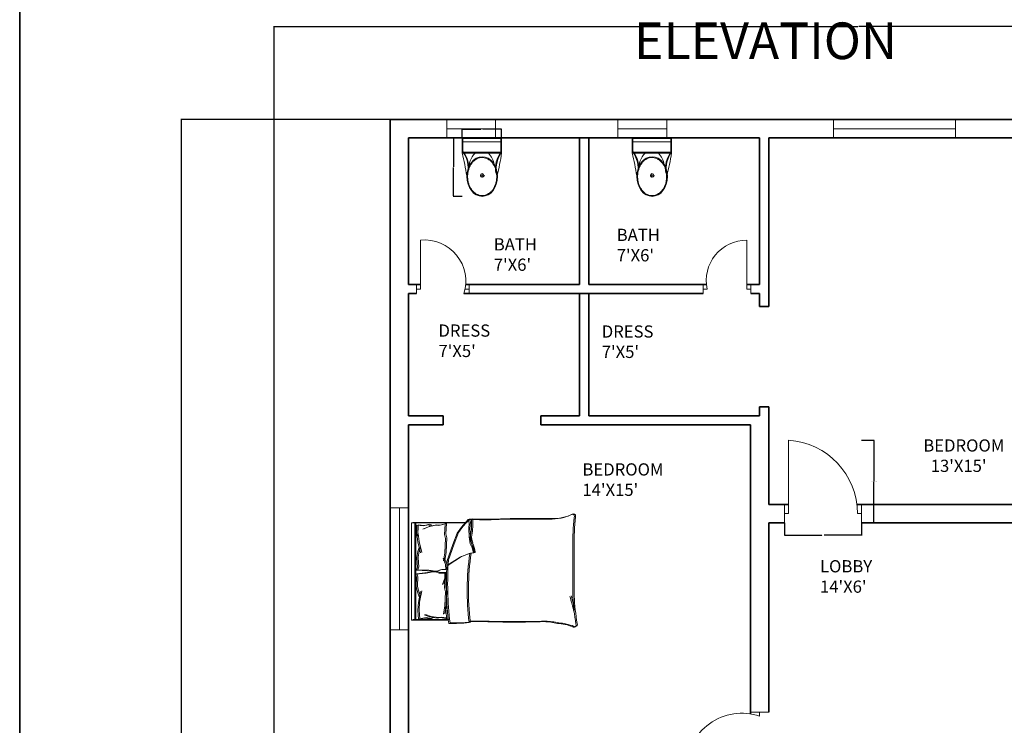
# Model space of a CAD drawing. Units: inches. Extents: x 1824 to 3509, y 619 to 2294.
# Tile 6 of 12: x 1824 to 2308, y 1325 to 1671. Entities that reach past the tile are written whole.
import ezdxf

# ---------------------------------------------------------------- set-up
doc = ezdxf.new("R2010")
doc.units = ezdxf.units.IN
for name, color, linetype, lineweight in [('A-ANNO-DIMS', 2, 'Continuous', 18), ('A-ANNO-TEXT', 7, 'Continuous', 25), ('A-ANNO-TTLB', 7, 'Continuous', 35), ('A-AREA-IDEN', 7, 'Continuous', 18), ('A-DOOR', 3, 'Continuous', 18), ('A-FLOR-FIXT', 9, 'Continuous', 18), ('A-FURN', 8, 'Continuous', 13), ('A-GLAZ', 4, 'Continuous', 18), ('A-WALL', 7, 'Continuous', 35)]:
    doc.layers.add(name, color=color, linetype=linetype, lineweight=lineweight)
doc.styles.get("Standard").update_dxf_attribs({"font": 'arial.ttf'})
doc.dimstyles.get("Standard").update_dxf_attribs({"dimtxt": 0.18, "dimasz": 0.18, "dimexe": 0.18, "dimexo": 0.0625, "dimgap": 0.09, "dimtad": 0, "dimtih": 1, "dimtoh": 1, "dimdec": 4, "dimzin": 0, "dimdsep": 46, "dimtxsty": 'Standard', "dimcen": 0.09, "dimadec": 0, "dimazin": 0, "dimtfac": 1, "dimtdec": 4, "dimtofl": 0, "dimtmove": 0, "dimatfit": 3, "dimfxl": 1, "dimtolj": 1, "dimtzin": 0, "dimarcsym": 0})

# ---------------------------------------------------------------- blocks, each defined once
blk = doc.blocks.new('A$C31115884')
for p, q in [((258, 466), (258, 523)), ((283, 498), (223, 498)), ((0, 200), (0, 0)), ((520, 200), (0, 200)), ((10, 190), (10, 10)), ((510, 190), (10, 190)), ((510, 10), (510, 190)), ((520, 0), (520, 200)), ((510, 54), (0, 54)), ((10, 10), (510, 10)), ((0, 0), (520, 0))]:
    blk.add_line(p, q)
blk.add_circle((256, 496), 23.6)
for centre, radius, start, end in [((2778, -205), 2807, 165.4549, 171.7133), ((-295, 403), 365, 324.2091, 9.3499), ((-295, 403), 375, 324.2091, 9.3499), ((139, 406), 293, 315.8436, 2.6563), ((806, 403), 375, 179.2036, 215.7909), ((806, 403), 365, 170.6501, 215.7909), ((3237, 905), 2807, 188.2867, 194.5451), ((384, 406), 293, 190.2774, 224.1564)]:
    blk.add_arc(centre, radius, start, end)
blk.add_ellipse((256, 510), major_axis=(0, -261), ratio=0.772727)
blk.add_open_spline([(256, 259), (263, 259), (270, 260), (288, 262), (299, 265), (320, 273), (330, 278), (350, 291), (360, 299), (378, 316), (386, 326), (402, 347), (409, 358), (421, 383), (427, 395), (436, 422), (440, 436), (445, 465), (447, 480), (448, 509), (448, 524), (445, 553), (443, 568), (436, 596), (432, 610), (422, 636), (416, 649), (402, 672), (395, 683), (379, 703), (370, 712), (351, 728), (341, 735), (321, 746), (310, 751), (289, 757), (278, 759), (256, 761), (245, 761), (223, 757), (212, 754), (191, 746), (181, 741), (161, 728), (151, 720), (133, 703), (125, 693), (110, 672), (103, 660), (90, 636), (85, 623), (76, 596), (72, 582), (67, 553), (66, 538), (64, 509), (65, 494), (68, 465), (70, 450), (77, 422), (81, 408), (91, 382), (97, 370), (111, 346), (118, 335), (135, 316), (144, 307), (162, 291), (172, 284), (193, 273), (203, 269), (225, 262), (236, 260), (250, 259), (253, 259), (256, 259)], degree=3, knots=[0, 0, 0, 0, 0.110105, 0.110105, 0.285049, 0.285049, 0.459994, 0.459994, 0.634938, 0.634938, 0.809882, 0.809882, 0.984827, 0.984827, 1.159771, 1.159771, 1.334715, 1.334715, 1.50966, 1.50966, 1.684604, 1.684604, 1.859549, 1.859549, 2.034493, 2.034493, 2.209437, 2.209437, 2.384382, 2.384382, 2.559326, 2.559326, 2.73427, 2.73427, 2.909215, 2.909215, 3.084159, 3.084159, 3.259103, 3.259103, 3.434048, 3.434048, 3.608992, 3.608992, 3.783936, 3.783936, 3.958881, 3.958881, 4.133825, 4.133825, 4.30877, 4.30877, 4.483714, 4.483714, 4.658658, 4.658658, 4.833603, 4.833603, 5.008547, 5.008547, 5.183491, 5.183491, 5.358436, 5.358436, 5.53338, 5.53338, 5.708324, 5.708324, 5.883269, 5.883269, 6.058213, 6.058213, 6.233158, 6.233158, 6.283185, 6.283185, 6.283185, 6.283185])
blk = doc.blocks.new('DOOR-BATH-W-24')
for p, q in [((2, 2.25), (2, 26.25)), ((0, 4.5), (0, 0)), ((0, 0), (0, 2.25)), ((0, 2.25), (2, 2.25)), ((25.84, 2.25), (23.84, 2.25)), ((25.84, 4.5), (25.84, 0)), ((25.84, 0), (25.84, 2.25))]:
    blk.add_line(p, q)
blk.add_arc((4.03, 6.16), 20.2, 342.2542, 95.7568)
blk = doc.blocks.new('DOOR-BATH-C-24')
for p, q in [((21.44, 2.25), (21.44, 26.25)), ((0, 4.5), (0, 0)), ((0, 0), (0, 2.25)), ((0, 2.25), (2, 2.25)), ((23.44, 2.25), (21.44, 2.25)), ((23.44, 4.5), (23.44, 0)), ((23.44, 0), (23.44, 2.25))]:
    blk.add_line(p, q)
blk.add_arc((21.44, 6.38), 19.87, 90, 191.9846)
blk = doc.blocks.new('DOOR-BED-W-36')
for p, q in [((31.5, 29.8), (40.5, 29.8)), ((40.5, 29.8), (36, 29.8)), ((36, 29.8), (36, 27.8)), ((36, 2), (0, 2)), ((31.5, 0), (31.5, 0)), ((31.5, 0), (40.5, 0)), ((36, 0), (36, 2)), ((40.5, 0), (36, 0)), ((36, 0), (36, 0)), ((40.5, 0), (40.5, 0))]:
    blk.add_line(p, q)
blk.add_arc((27.25, 2), 27.25, 71.2585, 180)
blk = doc.blocks.new('DOOR-BED-C-36')
for p, q in [((2, 4.5), (2, 40.5)), ((0, 9), (0, 0)), ((37.83, 9), (37.83, 9)), ((37.83, 9), (37.83, 0)), ((0, 0), (0, 4.5)), ((0, 4.5), (2, 4.5)), ((37.83, 4.5), (35.83, 4.5)), ((37.83, 0), (37.83, 4.5))]:
    blk.add_line(p, q)
blk.add_arc((-0.24, 4.5), 36.07, 0, 86.4439)
blk = doc.blocks.new('BED-DOUBLE-PLAN')
for p, q in [((0, 51.27), (26.61, 51.27)), ((0, 51.27), (26.61, 51.27)), ((0, 3.48), (0, 51.27)), ((0.64, 51.49), (27.25, 51.49)), ((0.64, 51.49), (27.25, 51.49)), ((1.53, 3.48), (1.53, 51.27)), ((1.53, 3.48), (1.53, 51.27)), ((2.17, 3.7), (2.17, 51.49)), ((2.17, 3.7), (2.17, 51.49)), ((2.56, 50.11), (2.46, 44.71)), ((2.56, 50.11), (2.46, 44.71)), ((2.56, 50.11), (5.77, 49.73)), ((2.56, 50.11), (5.77, 49.73)), ((3.2, 50.34), (3.1, 44.94)), ((3.2, 50.34), (3.1, 44.94)), ((3.2, 50.34), (6.41, 49.96)), ((3.2, 50.34), (6.41, 49.96)), ((8.26, 49.31), (5.58, 48.13)), ((8.26, 49.31), (5.58, 48.13)), ((5.77, 49.73), (8.34, 50.33)), ((5.77, 49.73), (8.34, 50.33)), ((8.9, 49.54), (6.22, 48.36)), ((8.9, 49.54), (6.22, 48.36)), ((6.41, 49.96), (8.98, 50.56)), ((6.41, 49.96), (8.98, 50.56)), ((11.83, 50.11), (8.26, 49.31)), ((11.83, 50.11), (8.26, 49.31)), ((8.34, 50.33), (9.38, 49.82)), ((8.34, 50.33), (9.38, 49.81)), ((12.47, 50.34), (8.9, 49.54)), ((12.47, 50.34), (8.9, 49.54)), ((8.98, 50.56), (10.02, 50.04)), ((8.98, 50.56), (10.02, 50.04)), ((13.43, 49.92), (11.83, 50.11)), ((13.43, 49.92), (11.83, 50.11)), ((14.07, 50.15), (12.47, 50.34)), ((14.07, 50.15), (12.47, 50.34)), ((16.57, 50.7), (13.43, 49.92)), ((16.57, 50.7), (13.43, 49.92)), ((17.21, 50.93), (14.07, 50.15)), ((17.21, 50.93), (14.07, 50.15)), ((16.17, 45.57), (16.57, 50.7)), ((16.17, 45.57), (16.57, 50.7)), ((16.81, 45.8), (17.21, 50.93)), ((16.81, 45.8), (17.21, 50.93)), ((24.5, 49.16), (22.33, 46.22)), ((24.5, 49.16), (22.33, 46.22)), ((25.13, 49.39), (22.97, 46.45)), ((25.13, 49.39), (22.97, 46.45)), ((27.75, 52.87), (24.5, 49.16)), ((27.75, 52.87), (24.5, 49.16)), ((28.39, 53.1), (25.13, 49.39)), ((28.39, 53.1), (25.13, 49.39)), ((29.49, 52.95), (27.75, 52.87, 3.87)), ((29.49, 52.95), (27.75, 52.87, 3.87)), ((28.36, 51.33), (27.75, 52.87)), ((28.36, 51.33), (27.75, 52.87)), ((28.06, 48.23), (28.36, 51.33)), ((28.06, 48.23), (28.36, 51.33)), ((30.13, 53.18), (28.39, 53.1, 3.87)), ((30.13, 53.18), (28.39, 53.1, 3.87)), ((29, 51.56), (28.39, 53.1)), ((29, 51.56), (28.39, 53.1)), ((28.69, 48.46), (29, 51.56)), ((28.69, 48.46), (29, 51.56)), ((29, 44.59), (28.69, 48.46)), ((29, 44.59), (28.69, 48.46)), ((2.46, 44.71), (2.54, 45.71)), ((2.46, 44.71), (2.54, 45.71)), ((2.54, 45.71), (3.07, 41.92)), ((2.54, 45.71), (3.07, 41.91)), ((3.1, 44.94), (3.18, 45.94)), ((3.1, 44.94), (3.18, 45.94)), ((3.18, 45.94), (3.71, 42.14)), ((3.18, 45.94), (3.71, 42.14)), ((16.73, 43.61), (16.17, 45.57)), ((16.73, 43.61), (16.17, 45.57)), ((16.3, 36.6), (16.73, 43.61)), ((16.3, 36.6), (16.73, 43.61)), ((17.37, 43.84), (16.81, 45.8)), ((17.37, 43.83), (16.81, 45.8)), ((16.93, 36.83), (17.37, 43.84)), ((16.93, 36.82), (17.37, 43.83)), ((22.33, 46.22), (20.32, 40.64)), ((22.33, 46.22), (20.32, 40.64)), ((22.97, 46.45), (20.96, 40.87)), ((22.97, 46.45), (20.96, 40.87)), ((28.36, 44.36), (28.06, 48.23)), ((28.36, 44.36), (28.06, 48.23)), ((28.83, 40.95), (28.36, 44.36)), ((28.83, 40.95), (28.36, 44.36)), ((29.47, 41.18), (29, 44.59)), ((29.47, 41.18), (29, 44.59)), ((3.07, 41.92), (4.42, 36.5)), ((3.07, 41.91), (4.42, 36.5)), ((3.67, 39.2), (3.08, 37.14)), ((3.67, 39.2), (3.08, 37.14)), ((3.71, 42.14), (5.06, 36.72)), ((3.71, 42.14), (5.06, 36.72)), ((4.31, 39.43), (3.72, 37.36)), ((4.31, 39.43), (3.72, 37.36)), ((20.32, 40.64), (17.38, 32.31)), ((20.32, 40.64), (17.38, 32.31)), ((20.96, 40.87), (18.02, 32.54)), ((20.96, 40.87), (18.02, 32.53)), ((29.76, 38.94), (28.83, 40.95)), ((29.76, 38.94), (28.83, 40.95)), ((30.4, 39.17), (29.47, 41.18)), ((30.4, 39.17), (29.47, 41.18)), ((30.38, 36.46), (29.76, 38.94)), ((30.38, 36.46), (29.76, 38.94)), ((31.02, 36.69), (30.4, 39.17)), ((31.02, 36.69), (30.4, 39.17)), ((79.24, 15.06), (79.24, 39.68)), ((79.24, 15.06), (79.24, 39.68)), ((79.88, 15.29), (79.88, 39.91)), ((79.88, 15.29), (79.88, 39.91)), ((3.08, 37.14), (2.54, 34.21)), ((3.08, 37.14), (2.54, 34.21)), ((2.54, 34.21), (2.56, 33.88)), ((2.54, 34.21), (2.56, 33.88)), ((2.56, 33.88), (2.98, 29.46)), ((2.56, 33.88), (2.98, 29.46)), ((3.72, 37.36), (3.18, 34.43)), ((3.72, 37.36), (3.18, 34.43)), ((3.18, 34.43), (3.2, 34.11)), ((3.18, 34.43), (3.2, 34.11)), ((3.2, 34.11), (3.62, 29.68)), ((3.2, 34.11), (3.62, 29.68)), ((15.63, 32.56), (16.3, 36.6)), ((15.63, 32.56), (16.3, 36.6)), ((17.38, 30.98), (16.09, 34.05)), ((17.38, 30.98), (16.09, 34.05)), ((16.27, 32.79), (16.93, 36.83)), ((16.27, 32.79), (16.93, 36.82)), ((17.38, 30.26), (23.88, 34.45)), ((17.38, 30.26), (23.88, 34.45)), ((18.02, 30.49), (24.52, 34.68)), ((18.02, 30.49), (24.52, 34.68)), ((23.88, 34.45), (28.36, 36.15)), ((23.88, 34.45), (28.36, 36.15)), ((24.52, 34.68), (29, 36.38)), ((24.52, 34.68), (29, 36.38)), ((28.36, 36.15), (30.38, 36.46)), ((28.36, 36.15), (30.38, 36.46)), ((29, 36.38), (31.02, 36.69)), ((29, 36.38), (31.02, 36.69)), ((2.98, 29.46), (2.49, 27.98)), ((2.98, 29.46), (2.49, 27.98)), ((3.62, 29.68), (3.13, 28.21)), ((3.62, 29.68), (3.13, 28.21)), ((16.74, 30.75), (15.45, 33.82)), ((16.74, 30.75), (15.45, 33.82)), ((16.89, 28.3), (16.74, 30.75)), ((16.89, 28.3), (16.74, 30.75)), ((17.53, 28.53), (17.38, 30.98)), ((17.53, 28.53), (17.38, 30.98)), ((1.87, 25.98), (7.22, 26.56)), ((1.87, 25.98), (7.22, 26.56)), ((2.45, 24.54), (1.87, 25.98)), ((2.45, 24.54), (1.87, 25.98)), ((2.3, 20.09), (2.45, 24.54)), ((2.3, 20.09), (2.45, 24.54)), ((2.49, 27.98), (7.87, 27.73)), ((2.49, 27.98), (7.87, 27.73)), ((2.51, 26.21), (7.86, 26.79)), ((2.51, 26.21), (7.86, 26.79)), ((3.09, 24.77), (2.51, 26.21)), ((3.09, 24.77), (2.51, 26.21)), ((2.94, 20.32), (3.09, 24.77)), ((2.94, 20.32), (3.09, 24.77)), ((3.13, 28.21), (8.51, 27.96)), ((3.13, 28.21), (8.51, 27.96)), ((7.22, 26.56), (10.4, 27.14)), ((7.22, 26.56), (10.4, 27.14)), ((7.86, 26.79), (11.04, 27.37)), ((7.86, 26.79), (11.04, 27.37)), ((7.87, 27.73), (11.08, 27.36)), ((7.87, 27.73), (11.08, 27.36)), ((8.51, 27.96), (11.72, 27.58)), ((8.51, 27.96), (11.72, 27.58)), ((10.4, 27.14), (11.7, 27.14)), ((10.4, 27.14), (11.7, 27.14)), ((11.04, 27.37), (12.34, 27.37)), ((11.04, 27.37), (12.34, 27.37)), ((11.08, 27.36), (12.38, 27.44)), ((11.08, 27.36), (12.38, 27.44)), ((11.7, 27.14), (13.58, 26.56)), ((11.7, 27.14), (13.58, 26.56)), ((11.72, 27.58), (13.02, 27.67)), ((11.72, 27.58), (13.02, 27.66)), ((12.34, 27.37), (14.22, 26.79)), ((12.34, 27.37), (14.22, 26.79)), ((12.38, 27.44), (14.22, 28.13)), ((12.38, 27.44), (14.22, 28.13)), ((13.02, 27.67), (14.86, 28.36)), ((13.02, 27.66), (14.86, 28.36)), ((13.58, 26.56), (16.26, 26.56)), ((13.58, 26.56), (16.26, 26.56)), ((14.22, 28.13), (16.89, 28.3)), ((14.22, 28.13), (16.89, 28.3)), ((14.22, 26.79), (16.9, 26.79)), ((14.22, 26.79), (16.9, 26.79)), ((14.86, 28.36), (17.53, 28.53)), ((14.86, 28.36), (17.53, 28.53)), ((16.9, 24.33), (15.81, 21.19)), ((16.9, 24.33), (15.81, 21.19)), ((16.17, 19.38), (16.57, 24.52)), ((16.17, 19.38), (16.57, 24.52)), ((16.26, 26.56), (16.26, 24.1)), ((16.26, 26.56), (16.26, 24.1)), ((16.81, 19.61), (17.21, 24.74)), ((16.81, 19.61), (17.21, 24.74)), ((16.9, 26.79), (16.9, 24.33)), ((16.9, 26.79), (16.9, 24.33)), ((2.3, 19.77), (2.3, 20.09)), ((2.3, 19.77), (2.3, 20.09)), ((3.03, 16.88), (2.3, 19.77)), ((3.03, 16.88), (2.3, 19.77)), ((2.94, 20), (2.94, 20.32)), ((2.94, 20), (2.94, 20.32)), ((3.67, 17.11), (2.94, 20)), ((3.67, 17.11), (2.94, 20)), ((16.26, 24.1), (15.17, 20.96)), ((16.26, 24.1), (15.17, 20.96)), ((16.73, 17.42), (16.17, 19.38)), ((16.73, 17.42), (16.17, 19.38)), ((17.37, 17.65), (16.81, 19.61)), ((17.37, 17.65), (16.81, 19.61)), ((3.75, 14.86), (3.03, 16.88)), ((3.75, 14.86), (3.03, 16.88)), ((3.32, 12.11), (4.33, 17.6)), ((3.32, 12.11), (4.33, 17.6)), ((4.39, 15.08), (3.67, 17.11)), ((4.39, 15.08), (3.67, 17.11)), ((3.96, 12.34), (4.97, 17.83)), ((3.96, 12.34), (4.97, 17.83)), ((16.3, 10.41), (16.73, 17.42)), ((16.3, 10.41), (16.73, 17.42)), ((16.93, 10.64), (17.37, 17.65)), ((16.93, 10.64), (17.37, 17.65)), ((3.03, 8.29), (3.32, 12.11)), ((3.03, 8.29), (3.32, 12.11)), ((3.67, 8.51), (3.96, 12.34)), ((3.67, 8.51), (3.96, 12.34)), ((15.63, 6.38), (16.3, 10.41)), ((15.63, 6.38), (16.3, 10.41)), ((16.27, 6.61), (16.93, 10.64)), ((16.27, 6.61), (16.93, 10.64)), ((16.3, 10.41), (16.62, 9.28)), ((16.3, 10.41), (16.62, 9.28)), ((16.93, 10.64), (17.26, 9.51)), ((16.93, 10.64), (17.26, 9.51)), ((3.01, 8.18), (3.03, 8.29)), ((3.01, 8.18), (3.03, 8.29)), ((3.34, 3.9), (3.01, 8.18)), ((3.34, 3.9), (3.01, 8.18)), ((3.65, 8.41), (3.67, 8.51)), ((3.65, 8.41), (3.67, 8.51)), ((3.98, 4.13), (3.65, 8.41)), ((3.98, 4.13), (3.65, 8.41)), ((8.95, 5.05), (6.21, 6.06)), ((8.95, 5.05), (6.21, 6.06)), ((9.59, 5.28), (6.85, 6.29)), ((9.59, 5.28), (6.85, 6.29)), ((12.57, 4.47), (8.95, 5.05)), ((12.57, 4.47), (8.95, 5.05)), ((13.21, 4.7), (9.59, 5.28)), ((13.21, 4.7), (9.59, 5.28)), ((9.74, 4.27), (10.75, 4.85)), ((9.74, 4.27), (10.75, 4.85)), ((14.8, 4.99), (13.21, 4.7)), ((14.8, 4.99), (13.21, 4.7)), ((17.98, 4.41), (14.8, 4.99)), ((17.98, 4.41), (14.8, 4.99)), ((16.62, 9.28), (17.34, 4.18)), ((16.62, 9.28), (17.34, 4.18)), ((17.26, 9.51), (17.98, 4.41)), ((17.26, 9.51), (17.98, 4.41)), ((18.11, 3.48), (0, 3.48)), ((18.11, 3.48), (0, 3.48)), ((18.75, 3.7), (0.64, 3.7)), ((18.75, 3.7), (0.64, 3.7)), ((3.32, 3.9), (6.5, 4.47)), ((3.32, 3.9), (6.5, 4.47)), ((3.96, 4.12), (7.14, 4.7)), ((3.96, 4.12), (7.14, 4.7)), ((6.5, 4.47), (9.1, 4.04)), ((6.5, 4.47), (9.1, 4.04)), ((7.14, 4.7), (9.74, 4.27)), ((7.14, 4.7), (9.74, 4.27)), ((9.1, 4.04), (10.11, 4.62)), ((9.1, 4.04), (10.11, 4.62)), ((14.16, 4.76), (12.57, 4.47)), ((14.16, 4.76), (12.57, 4.47)), ((17.34, 4.18), (14.16, 4.76)), ((17.34, 4.18), (14.16, 4.76))]:
    blk.add_line(p, q)
for centre, radius, start, end in [((36.95, 182.49), 129.5, 266.9791, 273.8365), ((36.95, 182.49), 129.5, 266.9791, 273.8365), ((68.46, -4508.51), 4561.86, 90.00217, 90.28689), ((68.46, -4508.51), 4561.86, 90.00217, 90.28689), ((68.67, 76.16), 23.07, 267.4714, 296.4681), ((68.67, 76.16), 23.07, 267.4714, 296.4681), ((69.31, 76.39), 23.07, 267.4714, 296.4681), ((69.31, 76.39), 23.07, 267.4714, 296.4681), ((78.87, 54.41), 1.1, 332.6588, 86.02), ((78.87, 54.41), 1.1, 332.6588, 86.02), ((212.28, 41.15), 133.04, 174.4998, 180.6351), ((212.28, 41.15), 133.04, 174.4998, 180.6351), ((79.51, 54.64), 1.1, 332.6588, 86.02), ((79.51, 54.64), 1.1, 332.6588, 86.02), ((212.92, 41.38), 133.04, 174.4998, 180.6351), ((212.92, 41.38), 133.04, 174.4998, 180.6351), ((-6.66, 51.33), 36.18, 349.8763, 2.5657), ((-6.66, 51.33), 36.18, 349.8763, 2.5657), ((36.32, 182.27), 129.5, 266.9791, 273.8365), ((36.32, 182.27), 129.5, 266.9791, 273.8365), ((-6.02, 51.56), 36.18, 349.8763, 2.5657), ((-6.02, 51.56), 36.18, 349.8763, 2.5657), ((67.82, -4508.74), 4561.86, 90.00217, 90.28689), ((67.82, -4508.74), 4561.86, 90.00217, 90.28689), ((35.07, 43.74), 6.22, 168.6608, 203.7384), ((35.07, 43.74), 6.22, 168.6608, 203.7384), ((35.71, 43.97), 6.22, 168.6608, 203.7384), ((35.71, 43.97), 6.22, 168.6608, 203.7384), ((1.48, 31.15), 29.65, 10.6617, 19.8806), ((1.48, 31.15), 29.65, 10.6617, 19.8806), ((2.12, 31.38), 29.65, 10.6617, 19.8806), ((2.12, 31.38), 29.65, 10.6617, 19.8806), ((156.32, 17.76), 129.02, 171.7845, 186.9006), ((156.32, 17.76), 129.02, 171.7845, 186.9006), ((156.96, 17.98), 129.02, 171.7845, 186.9006), ((156.96, 17.98), 129.02, 171.7845, 186.9006), ((30.44, 36.64), 0.185, 250.2464, 1.1377), ((30.44, 36.64), 0.185, 250.2464, 1.1377), ((31.08, 36.87), 0.185, 250.2464, 1.1377), ((31.08, 36.87), 0.185, 250.2464, 1.1377), ((182.05, 21.36), 164.97, 176.0865, 186.7821), ((182.05, 21.36), 164.97, 176.0865, 186.7821), ((182.69, 21.59), 164.97, 176.0865, 186.7821), ((182.69, 21.59), 164.97, 176.0865, 186.7821), ((-23.71, -17.22), 106.46, 13.3832, 17.7053), ((-23.71, -17.22), 106.46, 13.3832, 17.7053), ((-23.07, -16.99), 106.46, 13.3832, 17.7053), ((-23.07, -16.99), 106.46, 13.3832, 17.7053), ((200.84, 21.43), 121.76, 182.9958, 189.4091), ((200.84, 21.43), 121.76, 182.9958, 189.4091), ((201.48, 21.66), 121.76, 182.9958, 189.4091), ((201.48, 21.66), 121.76, 182.9958, 189.4091), ((20.1, 85.16), 83.31, 268.7218, 275.604), ((20.1, 85.16), 83.31, 268.7218, 275.604), ((20.74, 85.39), 83.31, 268.7218, 275.604), ((20.74, 85.39), 83.31, 268.7218, 275.604), ((31.17, -167.31), 170.11, 88.4762, 91.0082), ((31.17, -167.31), 170.11, 88.4762, 91.0082), ((31.81, -167.08), 170.11, 88.4762, 91.0082), ((31.81, -167.08), 170.11, 88.4762, 91.0082), ((50.61, 484.82), 482.31, 268.2277, 271.7185), ((50.61, 484.82), 482.31, 268.2277, 271.7185), ((51.25, 485.05), 482.31, 268.2277, 271.7185), ((51.25, 485.05), 482.31, 268.2277, 271.7185), ((64.52, -26.9), 29.63, 76.0648, 88.9113), ((64.52, -26.9), 29.63, 76.0648, 88.9113), ((65.15, -26.67), 29.63, 76.0648, 88.9113), ((65.15, -26.67), 29.63, 76.0648, 88.9113), ((70.28, -21.66), 23.56, 67.9751, 86.652), ((70.28, -21.66), 23.56, 67.9751, 86.652), ((70.91, -21.43), 23.56, 67.9751, 86.652), ((70.91, -21.43), 23.56, 67.9751, 86.652), ((79.72, 1.09), 1.09, 236.1736, 23.4781), ((79.72, 1.09), 1.09, 236.1736, 23.4781), ((80.36, 1.32), 1.09, 236.1736, 23.4781), ((80.36, 1.32), 1.09, 236.1736, 23.4781)]:
    blk.add_arc(centre, radius, start, end)
blk = doc.blocks.new('WIN-24')
for p, q in [((0, 0), (0, 9)), ((0, 9), (0, 4.5)), ((24, 0), (24, 9)), ((0, 4.5), (24, 4.5)), ((24, 4.5), (24, 0))]:
    blk.add_line(p, q)
blk = doc.blocks.new('WIN-60')
for p, q in [((0, 9), (0, 0)), ((60, 4.5), (60, 9)), ((60, 9), (60, 0)), ((0, 0), (0, 4.5)), ((0, 4.5), (60, 4.5))]:
    blk.add_line(p, q)
blk = doc.blocks.new('WIN-60-SIDE')
for p, q in [((9, 60), (0, 60)), ((0, 60), (4.5, 60)), ((4.5, 60), (4.5, 0)), ((4.5, 0), (0, 0)), ((0, 0), (9, 0))]:
    blk.add_line(p, q)
blk = doc.blocks.new('WIN-24-TOP')
for p, q in [((0, 0), (0, 9)), ((0, 9), (0, 4.5)), ((24, 4.5), (24, 9)), ((24, 9), (24, 0)), ((0, 4.5), (24, 4.5))]:
    blk.add_line(p, q)
blk = doc.blocks.new('*D40')
at = {"layer": 'A-ANNO-DIMS', "color": 0, "lineweight": -2, "transparency": 16777216}
for p, q in [((2041.38, 1613.1), (2036.95, 1613.1)), ((2037.13, 1612.92), (2037.13, 1598.92)), ((2037.13, 1584.56), (2037.13, 1598.56)), ((2041.38, 1584.38), (2036.95, 1584.38))]:
    blk.add_line(p, q, dxfattribs=at)
at = {"layer": 'A-ANNO-DIMS', "color": 0, "transparency": 16777216}
for points in [[(2037.1, 1612.92), (2037.16, 1612.92), (2037.13, 1613.1)], [(2037.1, 1584.56), (2037.16, 1584.56), (2037.13, 1584.38)]]:
    blk.add_solid(points, dxfattribs=at)
at = {"layer": 'Defpoints', "color": 0, "transparency": 16777216}
for p in [(2041.44, 1613.1), (2037.13, 1584.38), (2041.44, 1584.38)]:
    blk.add_point(p, dxfattribs=at)
at = {"layer": 'A-ANNO-DIMS', "color": 0, "transparency": 16777216, "insert": (2037.13, 1598.74), "char_height": 0.18, "attachment_point": 5}
blk.add_mtext('\\A1;WC 29 TYP.', dxfattribs=at)
blk = doc.blocks.new('*D41')
at = {"layer": 'A-ANNO-DIMS', "color": 0, "lineweight": -2, "transparency": 16777216}
for p, q in [((2041.44, 1613.16), (2041.44, 1617.59)), ((2041.62, 1617.41), (2050.61, 1617.41)), ((2060.64, 1617.41), (2051.65, 1617.41)), ((2060.82, 1613.16), (2060.82, 1617.59))]:
    blk.add_line(p, q, dxfattribs=at)
at = {"layer": 'A-ANNO-DIMS', "color": 0, "transparency": 16777216}
for points in [[(2041.62, 1617.44), (2041.62, 1617.38), (2041.44, 1617.41)], [(2060.64, 1617.44), (2060.64, 1617.38), (2060.82, 1617.41)]]:
    blk.add_solid(points, dxfattribs=at)
at = {"layer": 'Defpoints', "color": 0, "transparency": 16777216}
for p in [(2041.44, 1617.41), (2041.44, 1613.1), (2060.82, 1613.1)]:
    blk.add_point(p, dxfattribs=at)
at = {"layer": 'A-ANNO-DIMS', "color": 0, "transparency": 16777216, "insert": (2051.13, 1617.41), "char_height": 0.18, "attachment_point": 5}
blk.add_mtext('\\A1;19 TYP.', dxfattribs=at)
blk = doc.blocks.new('*D62')
at = {"layer": 'A-ANNO-DIMS', "color": 0, "lineweight": -2, "transparency": 16777216}
for p, q in [((2237.7, 1464.6), (2243.89, 1464.6)), ((2243.71, 1464.42), (2243.71, 1444.53)), ((2243.71, 1424.28), (2243.71, 1444.17)), ((2237.7, 1424.1), (2243.89, 1424.1))]:
    blk.add_line(p, q, dxfattribs=at)
at = {"layer": 'A-ANNO-DIMS', "color": 0, "transparency": 16777216}
for points in [[(2243.68, 1464.42), (2243.74, 1464.42), (2243.71, 1464.6)], [(2243.68, 1424.28), (2243.74, 1424.28), (2243.71, 1424.1)]]:
    blk.add_solid(points, dxfattribs=at)
at = {"layer": 'Defpoints', "color": 0, "transparency": 16777216}
for p in [(2237.63, 1464.6), (2243.71, 1464.6), (2237.63, 1424.1)]:
    blk.add_point(p, dxfattribs=at)
at = {"layer": 'A-ANNO-DIMS', "color": 0, "transparency": 16777216, "insert": (2243.71, 1444.35), "char_height": 0.18, "attachment_point": 5}
blk.add_mtext('\\A1;BEDROOM DOOR 41 TYP.', dxfattribs=at)
blk = doc.blocks.new('*D63')
at = {"layer": 'A-ANNO-DIMS', "color": 0, "lineweight": -2, "transparency": 16777216}
for p, q in [((2199.8, 1424.04), (2199.8, 1417.85)), ((2237.63, 1424.04), (2237.63, 1417.85)), ((2199.98, 1418.03), (2218.19, 1418.03)), ((2237.45, 1418.03), (2219.25, 1418.03))]:
    blk.add_line(p, q, dxfattribs=at)
at = {"layer": 'A-ANNO-DIMS', "color": 0, "transparency": 16777216}
for points in [[(2199.98, 1418.06), (2199.98, 1418), (2199.8, 1418.03)], [(2237.45, 1418.06), (2237.45, 1418), (2237.63, 1418.03)]]:
    blk.add_solid(points, dxfattribs=at)
at = {"layer": 'Defpoints', "color": 0, "transparency": 16777216}
for p in [(2199.8, 1424.1), (2237.63, 1424.1), (2237.63, 1418.03)]:
    blk.add_point(p, dxfattribs=at)
at = {"layer": 'A-ANNO-DIMS', "color": 0, "transparency": 16777216, "insert": (2218.72, 1418.03), "char_height": 0.18, "attachment_point": 5}
blk.add_mtext('\\A1;38 TYP.', dxfattribs=at)
blk = doc.blocks.new('*D94')
at = {"layer": 'A-ANNO-DIMS', "color": 0, "lineweight": -2, "transparency": 16777216}
for p, q in [((1949.09, 1049.16), (1949.09, 1668.03)), ((1949.27, 1667.85), (2235.8, 1667.85)), ((2522.91, 1667.85), (2236.38, 1667.85)), ((2523.09, 1622.16), (2523.09, 1668.03))]:
    blk.add_line(p, q, dxfattribs=at)
at = {"layer": 'A-ANNO-DIMS', "color": 0, "transparency": 16777216}
for points in [[(1949.27, 1667.88), (1949.27, 1667.82), (1949.09, 1667.85)], [(2522.91, 1667.88), (2522.91, 1667.82), (2523.09, 1667.85)]]:
    blk.add_solid(points, dxfattribs=at)
at = {"layer": 'Defpoints', "color": 0, "transparency": 16777216}
for p in [(2523.09, 1667.85), (2523.09, 1622.1), (1949.09, 1049.1)]:
    blk.add_point(p, dxfattribs=at)
at = {"layer": 'A-ANNO-DIMS', "color": 0, "transparency": 16777216, "insert": (2236.09, 1667.85), "char_height": 0.18, "attachment_point": 5}
blk.add_mtext('\\A1;574', dxfattribs=at)
blk = doc.blocks.new('*D95')
at = {"layer": 'A-ANNO-DIMS', "color": 0, "lineweight": -2, "transparency": 16777216}
for p, q in [((2006.03, 1622.1), (1903.16, 1622.1)), ((1903.34, 1621.92), (1903.34, 1202.28)), ((1903.34, 782.28), (1903.34, 1201.92)), ((1949.03, 782.1), (1903.16, 782.1))]:
    blk.add_line(p, q, dxfattribs=at)
at = {"layer": 'A-ANNO-DIMS', "color": 0, "transparency": 16777216}
for points in [[(1903.31, 1621.92), (1903.37, 1621.92), (1903.34, 1622.1)], [(1903.31, 782.28), (1903.37, 782.28), (1903.34, 782.1)]]:
    blk.add_solid(points, dxfattribs=at)
at = {"layer": 'Defpoints', "color": 0, "transparency": 16777216}
for p in [(1903.34, 1622.1), (2006.09, 1622.1), (1949.09, 782.1)]:
    blk.add_point(p, dxfattribs=at)
at = {"layer": 'A-ANNO-DIMS', "color": 0, "transparency": 16777216, "insert": (1903.34, 1202.1), "char_height": 0.18, "attachment_point": 5}
blk.add_mtext('\\A1;840', dxfattribs=at)

msp = doc.modelspace()

# ---------------------------------------------------------------- linework, layer by layer
at = {"layer": 'A-ANNO-TTLB'}
msp.add_lwpolyline([(1824.0608, 2293.6614), (3509.3484, 2293.6614), (3509.3484, 619.4665), (1824.0608, 619.4665)], close=True, dxfattribs=at)
at = {"layer": 'A-GLAZ'}
msp.add_line((2117.9957, 1622.1012), (2117.9957, 1622.1012), dxfattribs=at)
at = {"layer": 'A-WALL'}
for p, q in [((2006.0899, 1622.1012), (2006.0899, 1283.1012)), ((2006.0899, 1622.1012), (2523.0899, 1622.1012)), ((2015.0899, 1613.1012), (2187.5899, 1613.1012)), ((2015.0899, 1613.1012), (2015.0899, 1541.1012)), ((2099.0899, 1613.1012), (2099.0899, 1541.1012)), ((2103.5899, 1613.1012), (2103.5899, 1541.1012)), ((2187.5899, 1613.1012), (2187.5899, 1541.1012)), ((2192.0899, 1613.1012), (2192.0899, 1536.6012)), ((2192.0899, 1613.1012), (2348.0899, 1613.1012)), ((2015.0899, 1541.1012), (2020.995, 1541.1012)), ((2043.149, 1541.1012), (2099.0899, 1541.1012)), ((2103.5899, 1541.1012), (2161.4346, 1541.1012)), ((2181.2191, 1541.1012), (2187.5899, 1541.1012)), ((2015.0899, 1536.6012), (2018.995, 1536.6012)), ((2015.0899, 1536.6012), (2015.0899, 1476.6012)), ((2042.256, 1536.6012), (2159.779, 1536.6012)), ((2099.0899, 1536.6012), (2099.0899, 1476.6012)), ((2103.5899, 1536.6012), (2103.5899, 1476.6012)), ((2183.2191, 1536.6012), (2187.5899, 1536.6012)), ((2187.5899, 1536.6012), (2187.5899, 1530.3011)), ((2192.0899, 1536.6012), (2192.0899, 1530.3011)), ((2187.5899, 1530.3011), (2187.5899, 1530.3011)), ((2187.5899, 1530.3011), (2192.0899, 1530.3011)), ((2187.5899, 1480.9642), (2192.0899, 1480.9642)), ((2187.5899, 1480.9642), (2187.5899, 1476.6012)), ((2192.0899, 1480.9642), (2192.0899, 1433.1012)), ((2015.0899, 1476.6012), (2032.1437, 1476.6012)), ((2032.1437, 1472.1012), (2032.1437, 1476.6012)), ((2080.0206, 1472.1012), (2080.0206, 1476.6012)), ((2080.0206, 1476.6012), (2099.0899, 1476.6012)), ((2103.5899, 1476.6012), (2187.5899, 1476.6012)), ((2015.0899, 1472.1012), (2032.1437, 1472.1012)), ((2015.0899, 1472.1012), (2015.0899, 1292.1012)), ((2032.1437, 1472.1012), (2032.1437, 1472.1012)), ((2080.0206, 1472.1012), (2183.0899, 1472.1012)), ((2183.0899, 1472.1012), (2183.0899, 1330.1752)), ((2192.0899, 1433.1012), (2201.8012, 1433.1012)), ((2235.3516, 1433.1012), (2348.0899, 1433.1012)), ((2192.0899, 1424.1012), (2199.8012, 1424.1012)), ((2192.0899, 1424.1012), (2192.0899, 1331.0647)), ((2237.6334, 1424.1012), (2348.0899, 1424.1012))]:
    msp.add_line(p, q, dxfattribs=at)

# ---------------------------------------------------------------- block references
at = {"layer": 'A-DOOR'}
for name, p in [('DOOR-BATH-W-24', (2018.995, 1536.601)), ('DOOR-BATH-C-24', (2159.779, 1536.601)), ('DOOR-BED-C-36', (2199.801, 1424.101)), ('DOOR-BED-W-36', (2151.59, 1301.263))]:
    msp.add_blockref(name, p, dxfattribs=at)
at = {"layer": 'A-FLOR-FIXT', "xscale": 0.0372717239612423, "yscale": 0.0372717239612423, "zscale": 0.0372717239612423, "rotation": 180}
for p in [(2060.82, 1613.1012), (2144.318, 1613.1012)]:
    msp.add_blockref('A$C31115884', p, dxfattribs=at)
at = {"layer": 'A-FURN'}
msp.add_blockref('BED-DOUBLE-PLAN', (2016.59, 1372.794), dxfattribs=at)
at = {"layer": 'A-GLAZ'}
for name, p in [('WIN-24', (2033.897, 1613.101)), ('WIN-24-TOP', (2117.996, 1613.101)), ('WIN-60', (2223.859, 1613.101)), ('WIN-60-SIDE', (2006.09, 1371.438))]:
    msp.add_blockref(name, p, dxfattribs=at)

# ---------------------------------------------------------------- texts
at = {"layer": 'A-ANNO-TEXT', "insert": (2125.9029, 1669.7823), "char_height": 18, "attachment_point": 1}
msp.add_mtext_dynamic_manual_height_columns('ELEVATION', width=366.64266, gutter_width=12.5, heights=[0], dxfattribs=at)
at = {"layer": 'A-AREA-IDEN', "char_height": 6, "attachment_point": 1}
for s, width, insert in [("BATH\\P7'X6'", 44.719316, (2117.3725, 1568.4552)), ("BATH\\P7'X6'", 64.270001, (2056.9819, 1563.8095)), ("DRESS\\P7'X5'", 62.298858, (2029.7935, 1521.462)), ("DRESS\\P7'X5'", 84.606323, (2110.0129, 1521.0116)), ("BEDROOM\\P  13'X15'", 130.503843, (2267.9875, 1465.0376)), ("BEDROOM\\P14'X15'", 132.576713, (2100.5272, 1453.277)), ("LOBBY\\P14'X6'", 115.385501, (2217.2397, 1405.7145))]:
    msp.add_mtext_dynamic_manual_height_columns(s, width=width, gutter_width=12.5, heights=[0], dxfattribs=dict(at, insert=insert))

# ---------------------------------------------------------------- dimensions: what is measured, and where the dimension line sits
at = {"layer": 'A-ANNO-DIMS'}
dim = msp.add_linear_dim(base=(2523.0899, 1667.8512), p1=(1949.0899, 1049.1012), p2=(2523.0899, 1622.1012), dimstyle='Standard', override={"dimdec": 0, "dimlfac": 1, "dimrnd": 0, "dimzin": 0, "dimdsep": 46, "dimlunit": 2}, dxfattribs=at)
dim.commit()
dim.dimension.update_dxf_attribs({"geometry": '*D94', "text_midpoint": (2236.0899, 1667.8512)})
dim = msp.add_linear_dim(base=(1903.3399, 1622.1012), p1=(1949.0899, 782.1012), p2=(2006.0899, 1622.1012), angle=90, dimstyle='Standard', override={"dimdec": 0, "dimlfac": 1, "dimrnd": 0, "dimzin": 0, "dimdsep": 46, "dimlunit": 2}, dxfattribs=at)
dim.commit()
dim.dimension.update_dxf_attribs({"geometry": '*D95', "text_midpoint": (1903.3399, 1202.1012)})
for base, p1, p2, angle, text, picture, middle in [((2041.4387, 1617.4092), (2060.82, 1613.1012), (2041.4387, 1613.1012), 180, '<> TYP.', '*D41', (2051.1293, 1617.4092)), ((2037.1306, 1584.3807), (2041.4387, 1613.1012), (2041.4387, 1584.3807), 270, 'WC <> TYP.', '*D40', (2037.1306, 1598.7409)), ((2243.7083839323, 1464.6011662656), (2237.6333839323, 1424.1011662656), (2237.6333839323, 1464.6011662656), 90, 'BEDROOM DOOR <> TYP.', '*D62', (2243.7083839323, 1444.3511662656))]:
    dim = msp.add_linear_dim(base=base, p1=p1, p2=p2, angle=angle, text=text, dimstyle='Standard', override={"dimdec": 0, "dimlfac": 1, "dimrnd": 0, "dimzin": 0, "dimdsep": 46, "dimlunit": 2}, dxfattribs=at)
    dim.commit()
    dim.dimension.update_dxf_attribs({"geometry": picture, "text_midpoint": middle})
dim = msp.add_linear_dim(base=(2237.6334, 1418.0262), p1=(2199.8012, 1424.1012), p2=(2237.6334, 1424.1012), text='<> TYP.', dimstyle='Standard', override={"dimdec": 0, "dimlfac": 1, "dimrnd": 0, "dimzin": 0, "dimdsep": 46, "dimlunit": 2}, dxfattribs=at)
dim.commit()
dim.dimension.update_dxf_attribs({"geometry": '*D63', "text_midpoint": (2218.7173, 1418.0262)})

doc.saveas('drawing.dxf')
